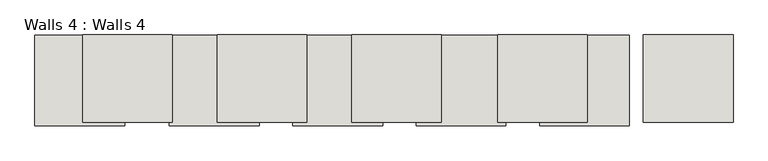
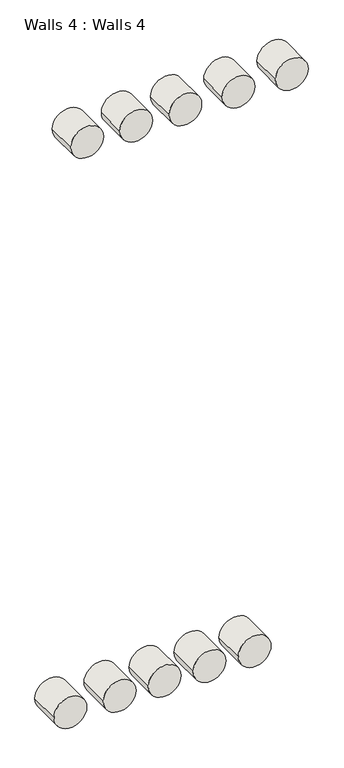
"""IFC4 building model written with IfcOpenShell, lengths in millimetres: wall geometry, Walls 4 : Walls 4."""

from ifc_helpers import new_model, si_unit, point, frame, frame_2d, origin, place, context, project, spatial, circle_curve, trimmed, segment, composite_curve, outline, extrude, source, transform, mapped, element, save


def walls_4_walls_4_cfa72774(model_context):
    return source(origin(), model_context, "Body", "SweptSolid", [
        extrude(outline(composite_curve([segment(trimmed(circle_curve(frame_2d((3793.9908284, -8701.5433714)), 101.6), [point((3793.9908284, -8803.1433714))], [point((3793.9908284, -8599.9433714))], False, "CARTESIAN"), True, "CONTINUOUS"), segment(trimmed(circle_curve(frame_2d((3793.9908284, -8701.5433714)), 101.6), [point((3793.9908284, -8599.9433714))], [point((3793.9908284, -8803.1433714))], False, "CARTESIAN"), True, "CONTINUOUS")], self_intersect=False)), frame((0.0, -1538.0653283, 0.0), z_axis=(0.0, 1.0, 0.0), x_axis=(0.0, 0.0, 1.0)), (0.0, 0.0, 1.0), 205.3757337),
        extrude(outline(composite_curve([segment(trimmed(circle_curve(frame_2d((3793.9908284, -8396.7433714)), 101.6), [point((3793.9908284, -8498.3433714))], [point((3793.9908284, -8295.1433714))], False, "CARTESIAN"), True, "CONTINUOUS"), segment(trimmed(circle_curve(frame_2d((3793.9908284, -8396.7433714)), 101.6), [point((3793.9908284, -8295.1433714))], [point((3793.9908284, -8498.3433714))], False, "CARTESIAN"), True, "CONTINUOUS")], self_intersect=False)), frame((0.0, -1538.0653283, 0.0), z_axis=(0.0, 1.0, 0.0), x_axis=(0.0, 0.0, 1.0)), (0.0, 0.0, 1.0), 205.3757337),
        extrude(outline(composite_curve([segment(trimmed(circle_curve(frame_2d((3793.9908284, -8117.3433714)), 101.6), [point((3793.9908284, -8218.9433714))], [point((3793.9908284, -8015.7433714))], False, "CARTESIAN"), True, "CONTINUOUS"), segment(trimmed(circle_curve(frame_2d((3793.9908284, -8117.3433714)), 101.6), [point((3793.9908284, -8015.7433714))], [point((3793.9908284, -8218.9433714))], False, "CARTESIAN"), True, "CONTINUOUS")], self_intersect=False)), frame((0.0, -1538.0653283, 0.0), z_axis=(0.0, 1.0, 0.0), x_axis=(0.0, 0.0, 1.0)), (0.0, 0.0, 1.0), 205.3757337),
        extrude(outline(composite_curve([segment(trimmed(circle_curve(frame_2d((3793.9908284, -7837.9433714)), 101.6), [point((3793.9908284, -7939.5433714))], [point((3793.9908284, -7736.3433714))], False, "CARTESIAN"), True, "CONTINUOUS"), segment(trimmed(circle_curve(frame_2d((3793.9908284, -7837.9433714)), 101.6), [point((3793.9908284, -7736.3433714))], [point((3793.9908284, -7939.5433714))], False, "CARTESIAN"), True, "CONTINUOUS")], self_intersect=False)), frame((0.0, -1538.0653283, 0.0), z_axis=(0.0, 1.0, 0.0), x_axis=(0.0, 0.0, 1.0)), (0.0, 0.0, 1.0), 205.3757337),
        extrude(outline(composite_curve([segment(trimmed(circle_curve(frame_2d((3793.9908284, -7558.5433714)), 101.6), [point((3793.9908284, -7660.1433714))], [point((3793.9908284, -7456.9433714))], False, "CARTESIAN"), True, "CONTINUOUS"), segment(trimmed(circle_curve(frame_2d((3793.9908284, -7558.5433714)), 101.6), [point((3793.9908284, -7456.9433714))], [point((3793.9908284, -7660.1433714))], False, "CARTESIAN"), True, "CONTINUOUS")], self_intersect=False)), frame((0.0, -1538.0653283, 0.0), z_axis=(0.0, 1.0, 0.0), x_axis=(0.0, 0.0, 1.0)), (0.0, 0.0, 1.0), 205.3757337),
        extrude(outline(composite_curve([segment(trimmed(circle_curve(frame_2d((7485.4728572, -8593.5325521)), 101.6), [point((7485.4728572, -8695.1325521))], [point((7485.4728572, -8491.9325521))], False, "CARTESIAN"), True, "CONTINUOUS"), segment(trimmed(circle_curve(frame_2d((7485.4728572, -8593.5325521)), 101.6), [point((7485.4728572, -8491.9325521))], [point((7485.4728572, -8695.1325521))], False, "CARTESIAN"), True, "CONTINUOUS")], self_intersect=False)), frame((0.0, -1530.0500552, 0.0), z_axis=(0.0, 1.0, 0.0), x_axis=(0.0, 0.0, 1.0)), (0.0, 0.0, 1.0), 197.3604606),
        extrude(outline(composite_curve([segment(trimmed(circle_curve(frame_2d((7485.4728572, -8288.7325521)), 101.6), [point((7485.4728572, -8390.3325521))], [point((7485.4728572, -8187.1325521))], False, "CARTESIAN"), True, "CONTINUOUS"), segment(trimmed(circle_curve(frame_2d((7485.4728572, -8288.7325521)), 101.6), [point((7485.4728572, -8187.1325521))], [point((7485.4728572, -8390.3325521))], False, "CARTESIAN"), True, "CONTINUOUS")], self_intersect=False)), frame((0.0, -1530.0500552, 0.0), z_axis=(0.0, 1.0, 0.0), x_axis=(0.0, 0.0, 1.0)), (0.0, 0.0, 1.0), 197.3604606),
        extrude(outline(composite_curve([segment(trimmed(circle_curve(frame_2d((7485.4728572, -7983.9325521)), 101.6), [point((7485.4728572, -8085.5325521))], [point((7485.4728572, -7882.3325521))], False, "CARTESIAN"), True, "CONTINUOUS"), segment(trimmed(circle_curve(frame_2d((7485.4728572, -7983.9325521)), 101.6), [point((7485.4728572, -7882.3325521))], [point((7485.4728572, -8085.5325521))], False, "CARTESIAN"), True, "CONTINUOUS")], self_intersect=False)), frame((0.0, -1530.0500552, 0.0), z_axis=(0.0, 1.0, 0.0), x_axis=(0.0, 0.0, 1.0)), (0.0, 0.0, 1.0), 197.3604606),
        extrude(outline(composite_curve([segment(trimmed(circle_curve(frame_2d((7485.4728572, -7653.7325521)), 101.6), [point((7485.4728572, -7755.3325521))], [point((7485.4728572, -7552.1325521))], False, "CARTESIAN"), True, "CONTINUOUS"), segment(trimmed(circle_curve(frame_2d((7485.4728572, -7653.7325521)), 101.6), [point((7485.4728572, -7552.1325521))], [point((7485.4728572, -7755.3325521))], False, "CARTESIAN"), True, "CONTINUOUS")], self_intersect=False)), frame((0.0, -1530.0500552, 0.0), z_axis=(0.0, 1.0, 0.0), x_axis=(0.0, 0.0, 1.0)), (0.0, 0.0, 1.0), 197.3604606),
        extrude(outline(composite_curve([segment(trimmed(circle_curve(frame_2d((7485.4728572, -7323.5325521)), 101.6), [point((7485.4728572, -7425.1325521))], [point((7485.4728572, -7221.9325521))], False, "CARTESIAN"), True, "CONTINUOUS"), segment(trimmed(circle_curve(frame_2d((7485.4728572, -7323.5325521)), 101.6), [point((7485.4728572, -7221.9325521))], [point((7485.4728572, -7425.1325521))], False, "CARTESIAN"), True, "CONTINUOUS")], self_intersect=False)), frame((0.0, -1530.0500552, 0.0), z_axis=(0.0, 1.0, 0.0), x_axis=(0.0, 0.0, 1.0)), (0.0, 0.0, 1.0), 197.3604606),
    ])


if __name__ == "__main__":
    model = new_model("IFC4")
    model_context = context("Model", 3, world=origin())
    ifc_project = project(units=[si_unit("LENGTHUNIT", "METRE", prefix="MILLI")], contexts=[model_context])
    site = spatial("IfcSite", under=ifc_project)
    building = spatial("IfcBuilding", under=site)
    placement = place(None, origin())
    walls_4_walls_4_shape = walls_4_walls_4_cfa72774(model_context)
    element("IfcWall", 1, ObjectType="Walls 4 : Walls 4", at=placement, inside=building, context=model_context, shape_type="MappedRepresentation", body=[
        mapped(walls_4_walls_4_shape, transform((0.0, 0.0, 0.0), x_axis=(1.0, 0.0, 0.0), y_axis=(0.0, 1.0, 0.0), z_axis=(0.0, 0.0, 1.0))),
    ])
    save(model, "model.ifc")

# Revit data of these elements
# Element 1 (IfcWall, "Walls 4 : Walls 4")
#   Materials on its faces: "Default Wall"
# Materials
#   "Default Wall": colour RGB 128 128 128, transparency 0
